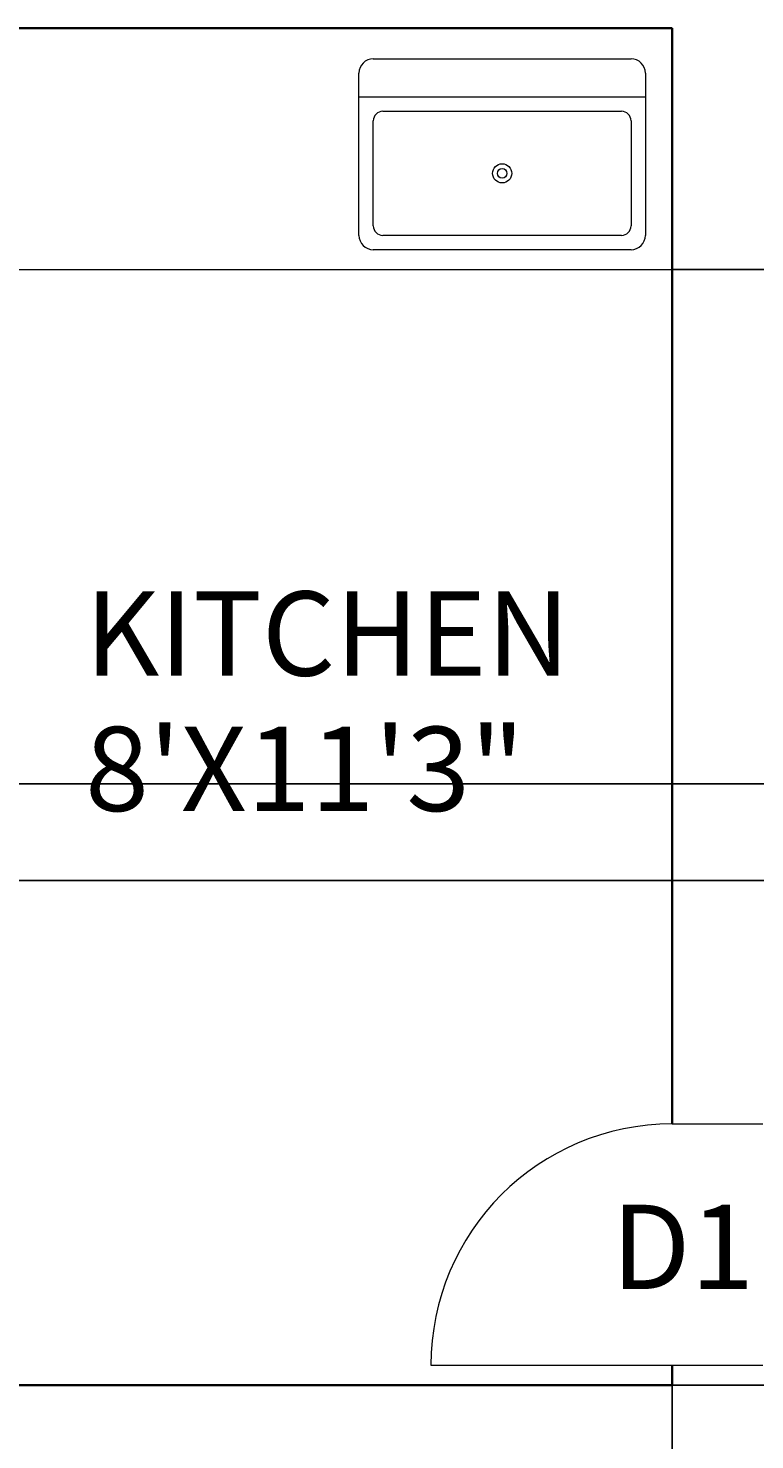
# Model space of a CAD drawing. Units: feet. Extents: x 1654 to 2985, y 1348 to 2230.
# Tile 7 of 53: x 1884 to 1956, y 1746 to 1886. Entities that reach past the tile are written whole.
import ezdxf

# ---------------------------------------------------------------- set-up
doc = ezdxf.new("R2010")
doc.units = ezdxf.units.FT
for name, color, linetype, lineweight in [('A-ANNO-DIMS', 2, 'Continuous', 18), ('A-ANNO-TEXT', 7, 'Continuous', 18), ('A-AREA-IDEN', 7, 'Continuous', 18), ('A-DOOR', 3, 'Continuous', 18), ('A-FLOR-CASE', 8, 'Continuous', 18), ('A-FLOR-FIXT', 8, 'Continuous', 18), ('A-WALL', 7, 'Continuous', 35)]:
    doc.layers.add(name, color=color, linetype=linetype, lineweight=lineweight)
doc.styles.get("Standard").update_dxf_attribs({"font": 'arial.ttf'})
doc.dimstyles.get("Standard").update_dxf_attribs({"dimtxt": 0.18, "dimasz": 0.18, "dimexe": 0.18, "dimexo": 0.0625, "dimgap": 0.09, "dimtad": 0, "dimtih": 1, "dimtoh": 1, "dimdec": 4, "dimzin": 0, "dimdsep": 46, "dimtxsty": 'Standard', "dimcen": 0.09, "dimadec": 0, "dimazin": 0, "dimtfac": 1, "dimtdec": 4, "dimtofl": 0, "dimtmove": 0, "dimatfit": 3, "dimfxl": 1, "dimtolj": 1, "dimtzin": 0, "dimarcsym": 0})

# ---------------------------------------------------------------- blocks, each defined once
blk = doc.blocks.new('Sink-single - 30 in top')
blk.add_line((-15, -3.999996), (15, -3.999996))
for points in [[(-13.5, 0), (13.5, 0)], [(-15, -18.499996), (-15, -1.5)], [(15, -1.5), (15, -18.499996)], [(-12.5, -5.499996), (12.5, -5.499996)], [(-13.5, -17.499996), (-13.5, -6.499996)], [(13.5, -6.499996), (13.5, -17.499996)], [(12.5, -18.499996), (-12.5, -18.499996)], [(13.5, -19.999996), (-13.5, -19.999996)]]:
    blk.add_lwpolyline(points)
for radius in [1, 0.5]:
    blk.add_circle((0, -11.999996), radius)
for centre, radius, start, end in [((-13.5, -1.5), 1.5, 90, 180), ((13.5, -1.5), 1.5, 0, 90), ((-12.5, -6.499996), 1, 90, 180), ((12.5, -6.499996), 1, 0, 90), ((-12.5, -17.499996), 1, 180, 270), ((12.5, -17.499996), 1, 270, 0), ((-13.5, -18.499996), 1.5, 180, 270), ((13.5, -18.499996), 1.5, 270, 0)]:
    blk.add_arc(centre, radius, start, end)
blk = doc.blocks.new('DOOR-INT-SINGLE')
for p, q in [((0, 24), (9, 24)), ((-24, 0), (9, 0))]:
    blk.add_line(p, q)
blk.add_arc((0, 0), 24, 90, 180)
blk = doc.blocks.new('CASEWORK-KITCHEN-L')
for q in [(72, 111), (0, 0)]:
    blk.add_line((0, 111), q)
blk = doc.blocks.new('*D74')
at = {"layer": 'A-ANNO-DIMS', "color": 0, "lineweight": -2, "transparency": 16777216}
for p, q in [((1948.15, 1862.25), (1964.92, 1862.25)), ((1964.74, 1862.07), (1964.74, 1806.94)), ((1964.74, 1751.43), (1964.74, 1806.57)), ((1948.15, 1751.25), (1964.92, 1751.25))]:
    blk.add_line(p, q, dxfattribs=at)
at = {"layer": 'A-ANNO-DIMS', "color": 0, "transparency": 16777216}
for points in [[(1964.71, 1862.07), (1964.77, 1862.07), (1964.74, 1862.25)], [(1964.71, 1751.43), (1964.77, 1751.43), (1964.74, 1751.25)]]:
    blk.add_solid(points, dxfattribs=at)
at = {"layer": 'Defpoints', "color": 0, "transparency": 16777216}
for p in [(1948.09, 1862.25), (1964.74, 1862.25), (1948.09, 1751.25)]:
    blk.add_point(p, dxfattribs=at)
at = {"layer": 'A-ANNO-DIMS', "color": 0, "transparency": 16777216, "insert": (1964.74, 1806.75), "char_height": 0.18, "attachment_point": 5}
blk.add_mtext('\\A1;COUNTER 111 TYP.', dxfattribs=at)
blk = doc.blocks.new('*D75')
at = {"layer": 'A-ANNO-DIMS', "color": 0, "lineweight": -2, "transparency": 16777216}
for p, q in [((1876.09, 1751.19), (1876.09, 1734.42)), ((1948.09, 1751.19), (1948.09, 1734.42)), ((1876.27, 1734.6), (1911.57, 1734.6)), ((1947.91, 1734.6), (1912.62, 1734.6))]:
    blk.add_line(p, q, dxfattribs=at)
at = {"layer": 'A-ANNO-DIMS', "color": 0, "transparency": 16777216}
for points in [[(1876.27, 1734.63), (1876.27, 1734.57), (1876.09, 1734.6)], [(1947.91, 1734.63), (1947.91, 1734.57), (1948.09, 1734.6)]]:
    blk.add_solid(points, dxfattribs=at)
at = {"layer": 'Defpoints', "color": 0, "transparency": 16777216}
for p in [(1876.09, 1751.25), (1948.09, 1751.25), (1948.09, 1734.6)]:
    blk.add_point(p, dxfattribs=at)
at = {"layer": 'A-ANNO-DIMS', "color": 0, "transparency": 16777216, "insert": (1912.09, 1734.6), "char_height": 0.18, "attachment_point": 5}
blk.add_mtext('\\A1;72 TYP.', dxfattribs=at)
blk = doc.blocks.new('*D91')
at = {"layer": 'A-ANNO-DIMS', "color": 0, "lineweight": -2, "transparency": 16777216}
for p, q in [((1852.15, 1801.47), (2242.27, 1801.47)), ((2242.09, 1801.29), (2242.09, 1776.54)), ((2242.09, 1751.43), (2242.09, 1776.18)), ((1852.15, 1751.25), (2242.27, 1751.25))]:
    blk.add_line(p, q, dxfattribs=at)
at = {"layer": 'A-ANNO-DIMS', "color": 0, "transparency": 16777216}
for points in [[(2242.06, 1801.29), (2242.12, 1801.29), (2242.09, 1801.47)], [(2242.06, 1751.43), (2242.12, 1751.43), (2242.09, 1751.25)]]:
    blk.add_solid(points, dxfattribs=at)
at = {"layer": 'Defpoints', "color": 0, "transparency": 16777216}
for p in [(1852.09, 1801.47), (2242.09, 1801.47), (1852.09, 1751.25)]:
    blk.add_point(p, dxfattribs=at)
at = {"layer": 'A-ANNO-DIMS', "color": 0, "transparency": 16777216, "insert": (2242.09, 1776.36), "char_height": 0.18, "attachment_point": 5}
blk.add_mtext('\\A1;50.21', dxfattribs=at)
blk = doc.blocks.new('*D98')
at = {"layer": 'A-ANNO-DIMS', "color": 0, "lineweight": -2, "transparency": 16777216}
for p, q in [((2061.03, 1811.08), (1811.91, 1811.08)), ((1812.09, 1810.9), (1812.09, 1781.35)), ((1812.09, 1751.43), (1812.09, 1780.99)), ((2061.03, 1751.25), (1811.91, 1751.25))]:
    blk.add_line(p, q, dxfattribs=at)
at = {"layer": 'A-ANNO-DIMS', "color": 0, "transparency": 16777216}
for points in [[(1812.06, 1810.9), (1812.12, 1810.9), (1812.09, 1811.08)], [(1812.06, 1751.43), (1812.12, 1751.43), (1812.09, 1751.25)]]:
    blk.add_solid(points, dxfattribs=at)
at = {"layer": 'Defpoints', "color": 0, "transparency": 16777216}
for p in [(1812.09, 1811.08), (2061.09, 1811.08), (2061.09, 1751.25)]:
    blk.add_point(p, dxfattribs=at)
at = {"layer": 'A-ANNO-DIMS', "color": 0, "transparency": 16777216, "insert": (1812.09, 1781.17), "char_height": 0.18, "attachment_point": 5}
blk.add_mtext('\\A1;59.83', dxfattribs=at)

msp = doc.modelspace()

# ---------------------------------------------------------------- linework, layer by layer
at = {"layer": 'A-WALL'}
for p, q in [((1852.0924, 1886.2549), (1948.0924, 1886.2549)), ((1948.0924, 1777.2549), (1948.0924, 1886.2549)), ((1948.0924, 1751.2549), (1948.0924, 1753.2549)), ((1852.0924, 1751.2549), (1948.0924, 1751.2549))]:
    msp.add_line(p, q, dxfattribs=at)

# ---------------------------------------------------------------- block references
at = {"layer": 'A-DOOR'}
msp.add_blockref('DOOR-INT-SINGLE', (1948.0924, 1753.2549), dxfattribs=at)
at = {"layer": 'A-FLOR-CASE'}
msp.add_blockref('CASEWORK-KITCHEN-L', (1876.092, 1751.255), dxfattribs=at)
at = {"layer": 'A-FLOR-FIXT', "xscale": 0.9494788357391524, "yscale": 0.9494788357391524, "zscale": 0.9494788357391524}
msp.add_blockref('Sink-single - 30 in top', (1931.181, 1883.2123), dxfattribs=at)

# ---------------------------------------------------------------- texts
at = {"layer": 'A-ANNO-TEXT'}
msp.add_text('D1', height=8.38114, dxfattribs=at).set_placement((1942.0453, 1760.8311))
at = {"layer": 'A-AREA-IDEN'}
for s, p in [('KITCHEN', (1889.7003, 1821.8452)), ('8\'X11\'3"', (1889.7003, 1808.3816))]:
    msp.add_text(s, height=8.38114, dxfattribs=at).set_placement(p)

# ---------------------------------------------------------------- dimensions: what is measured, and where the dimension line sits
at = {"layer": 'A-ANNO-DIMS'}
dim = msp.add_linear_dim(base=(1964.7424, 1862.2549), p1=(1948.0924, 1751.2549), p2=(1948.0924, 1862.2549), angle=90, text='COUNTER <> TYP.', dimstyle='Standard', override={"dimdec": 0, "dimlfac": 1, "dimrnd": 0, "dimzin": 0, "dimdsep": 46, "dimlunit": 2}, dxfattribs=at)
dim.commit()
dim.dimension.update_dxf_attribs({"geometry": '*D74', "text_midpoint": (1964.7424, 1806.7549)})
for base, p1, p2, picture, middle in [((1812.0924, 1811.0815), (2061.0924, 1751.2549), (2061.0924, 1811.0815), '*D98', (1812.0924, 1781.1682)), ((2242.0924, 1801.4683), (1852.0924, 1751.2549), (1852.0924, 1801.4683), '*D91', (2242.0924, 1776.3616))]:
    dim = msp.add_linear_dim(base=base, p1=p1, p2=p2, angle=90, dimstyle='Standard', override={"dimdec": 2, "dimlfac": 1, "dimrnd": 0, "dimzin": 0, "dimdsep": 46, "dimlunit": 2}, dxfattribs=at)
    dim.commit()
    dim.dimension.update_dxf_attribs({"geometry": picture, "text_midpoint": middle})
dim = msp.add_linear_dim(base=(1948.0924, 1734.6049), p1=(1876.0924, 1751.2549), p2=(1948.0924, 1751.2549), text='<> TYP.', dimstyle='Standard', override={"dimdec": 0, "dimlfac": 1, "dimrnd": 0, "dimzin": 0, "dimdsep": 46, "dimlunit": 2}, dxfattribs=at)
dim.commit()
dim.dimension.update_dxf_attribs({"geometry": '*D75', "text_midpoint": (1912.0924, 1734.6049)})

doc.saveas('drawing.dxf')
